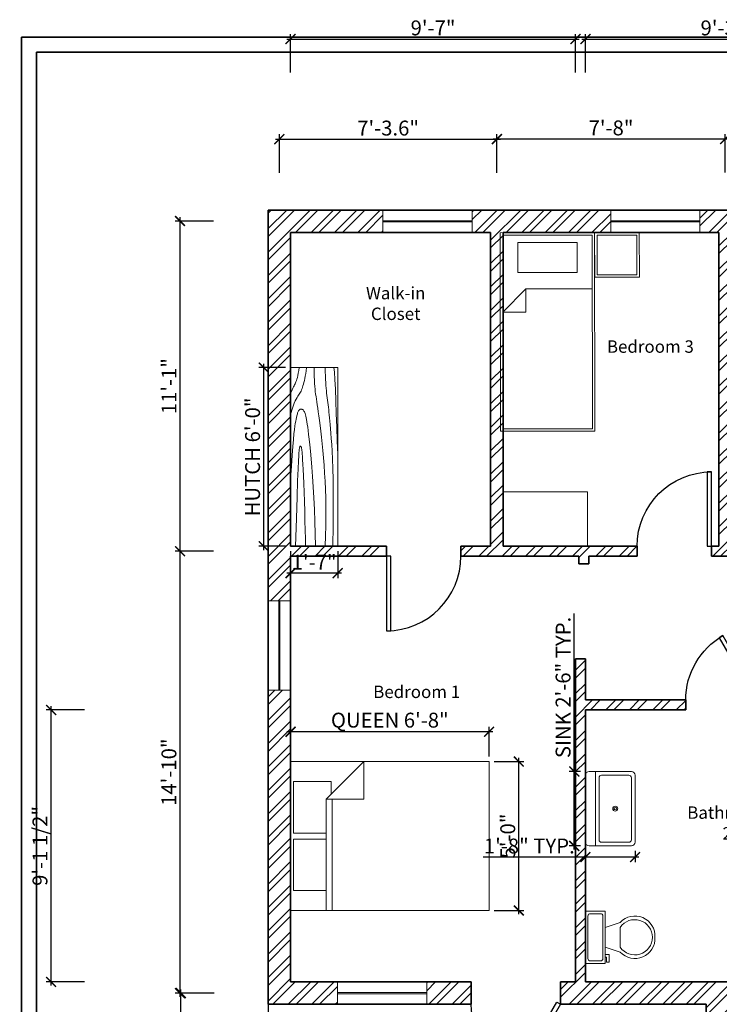
# Model space of a CAD drawing. Units: inches. Extents: x 163 to 947, y 159 to 804.
# Tile 2 of 5: x 163 to 444, y 403 to 799. Entities that reach past the tile are written whole.
import ezdxf

# ---------------------------------------------------------------- set-up
doc = ezdxf.new("R2010")
doc.units = ezdxf.units.IN
for name, color, linetype, lineweight in [('A-ANNO-TTLB', 7, 'Continuous', 35), ('A-AREA-IDEN', 7, 'Continuous', 18), ('A-FLOR-FIXT', 121, 'Continuous', 18), ('A-FLOR-OTLN', 7, 'Continuous', 25), ('Dimensions', 7, 'Continuous', 18), ('Doors', 160, 'Continuous', 25), ('Furniture', 40, 'Continuous', 18), ('Wall Hatch', 214, 'Continuous', 13), ('Walls', 222, 'Continuous', 35), ('Windows', 132, 'Continuous', 18)]:
    doc.layers.add(name, color=color, linetype=linetype, lineweight=lineweight)
doc.styles.get("Standard").update_dxf_attribs({"font": 'arial.ttf'})
doc.dimstyles.new('ISO-25', dxfattribs={"dimtxt": 6, "dimasz": 4, "dimexe": 2, "dimexo": 2, "dimtad": 1, "dimdec": 1, "dimlunit": 3, "dimtxsty": 'Standard', "dimblk": 'ARCHTICK', "dimcen": 0, "dimdle": 1.5, "dimadec": 0, "dimazin": 0, "dimtfac": 1, "dimtdec": 1, "dimtmove": 0, "dimatfit": 3, "dimfxl": 13.5, "dimfxlon": 1, "dimarcsym": 0})

# ---------------------------------------------------------------- blocks, each defined once
blk = doc.blocks.new('_ArchTick')
at = {"color": 0, "linetype": 'ByBlock', "const_width": 0.15}
blk.add_lwpolyline([(-0.5, -0.5), (0.5, 0.5)], dxfattribs=at)
blk = doc.blocks.new('*D6')
at = {"layer": 'Dimensions', "color": 0, "lineweight": -2, "transparency": 16777216}
for p, q in [((448.3, 751.36), (353.3, 751.36)), ((354.8, 737.86), (354.8, 753.36)), ((446.8, 737.86), (446.8, 753.36))]:
    blk.add_line(p, q, dxfattribs=at)
at = {"layer": 'Dimensions', "color": 0, "lineweight": -2, "transparency": 16777216, "xscale": 4, "yscale": 4, "zscale": 4, "rotation": 180}
blk.add_blockref('_ArchTick', (354.8, 751.36), dxfattribs=at)
at = {"layer": 'Dimensions', "color": 0, "lineweight": -2, "transparency": 16777216, "xscale": 4, "yscale": 4, "zscale": 4}
blk.add_blockref('_ArchTick', (446.8, 751.36), dxfattribs=at)
at = {"layer": 'Dimensions', "color": 0, "transparency": 16777216, "insert": (400.8, 755.05), "char_height": 6, "attachment_point": 5}
blk.add_mtext('7\'-8"', dxfattribs=at)
blk = doc.blocks.new('*D7')
at = {"layer": 'Dimensions', "color": 0, "lineweight": -2, "transparency": 16777216}
for p, q in [((265.66, 751.3), (356.3, 751.3)), ((267.16, 737.8), (267.16, 753.3)), ((354.8, 737.8), (354.8, 753.3))]:
    blk.add_line(p, q, dxfattribs=at)
at = {"layer": 'Dimensions', "color": 0, "lineweight": -2, "transparency": 16777216, "xscale": 4, "yscale": 4, "zscale": 4, "rotation": 180}
blk.add_blockref('_ArchTick', (267.16, 751.3), dxfattribs=at)
at = {"layer": 'Dimensions', "color": 0, "lineweight": -2, "transparency": 16777216, "xscale": 4, "yscale": 4, "zscale": 4}
blk.add_blockref('_ArchTick', (354.8, 751.3), dxfattribs=at)
at = {"layer": 'Dimensions', "color": 0, "transparency": 16777216, "insert": (310.98, 754.99), "char_height": 6, "attachment_point": 5}
blk.add_mtext('7\'-3.6"', dxfattribs=at)
blk = doc.blocks.new('*D15')
at = {"layer": 'Dimensions', "color": 0, "lineweight": -2, "transparency": 16777216}
for p, q in [((227.45, 288.78), (227.45, 408.78)), ((240.95, 407.28), (225.45, 407.28)), ((240.95, 290.28), (225.45, 290.28))]:
    blk.add_line(p, q, dxfattribs=at)
at = {"layer": 'Dimensions', "color": 0, "lineweight": -2, "transparency": 16777216, "xscale": 4, "yscale": 4, "zscale": 4}
for p, rotation in [((227.45, 407.28), 90), ((227.45, 290.28), 270)]:
    blk.add_blockref('_ArchTick', p, dxfattribs=dict(at, rotation=rotation))
at = {"layer": 'Dimensions', "color": 0, "transparency": 16777216, "insert": (223.76, 348.78), "char_height": 6, "attachment_point": 5, "rotation": 90}
blk.add_mtext('9\'-9"', dxfattribs=at)
blk = doc.blocks.new('*D16')
at = {"layer": 'Dimensions', "color": 0, "lineweight": -2, "transparency": 16777216}
for p, q in [((240.62, 585.28), (225.12, 585.28)), ((227.12, 405.78), (227.12, 586.78)), ((240.62, 407.28), (225.12, 407.28))]:
    blk.add_line(p, q, dxfattribs=at)
at = {"layer": 'Dimensions', "color": 0, "lineweight": -2, "transparency": 16777216, "xscale": 4, "yscale": 4, "zscale": 4}
for p, rotation in [((227.12, 585.28), 90), ((227.12, 407.28), 270)]:
    blk.add_blockref('_ArchTick', p, dxfattribs=dict(at, rotation=rotation))
at = {"layer": 'Dimensions', "color": 0, "transparency": 16777216, "insert": (223.43, 496.28), "char_height": 6, "attachment_point": 5, "rotation": 90}
blk.add_mtext('14\'-10"', dxfattribs=at)
blk = doc.blocks.new('*D17')
at = {"layer": 'Dimensions', "color": 0, "lineweight": -2, "transparency": 16777216}
for p, q in [((240.62, 718.32), (225.12, 718.32)), ((227.12, 583.78), (227.12, 719.82)), ((240.62, 585.28), (225.12, 585.28))]:
    blk.add_line(p, q, dxfattribs=at)
at = {"layer": 'Dimensions', "color": 0, "lineweight": -2, "transparency": 16777216, "xscale": 4, "yscale": 4, "zscale": 4}
for p, rotation in [((227.12, 718.32), 90), ((227.12, 585.28), 270)]:
    blk.add_blockref('_ArchTick', p, dxfattribs=dict(at, rotation=rotation))
at = {"layer": 'Dimensions', "color": 0, "transparency": 16777216, "insert": (223.48, 651.8), "char_height": 6, "attachment_point": 5, "rotation": 90}
blk.add_mtext('11\'-1"', dxfattribs=at)
blk = doc.blocks.new('*U19')
for p, q in [((0, 0), (0, 4)), ((30, 0), (30, 4))]:
    blk.add_line(p, q)
blk.add_lwpolyline([(0, 0), (0, -30), (1.75, -30), (1.75, 0)], close=True)
blk.add_arc((0, 0), 30, 270, 0)
blk = doc.blocks.new('*U20')
for p, q in [((0, 0), (0, -4)), ((30, 0), (30, -4))]:
    blk.add_line(p, q)
blk.add_lwpolyline([(0, 0), (0, 30), (1.75, 30), (1.75, 0)], close=True)
blk.add_arc((0, 0), 30, 0, 90)
blk = doc.blocks.new('*U21')
for p, q in [((0, 0), (0, -4)), ((30, 0), (30, -4))]:
    blk.add_line(p, q)
blk.add_lwpolyline([(0, 0), (15, 25.98), (16.52, 25.11), (1.52, -0.87)], close=True)
blk.add_arc((0, 0), 30, 0, 60)
blk = doc.blocks.new('*U22')
for p, q in [((0, 0), (0, 6)), ((36, 0), (36, 6))]:
    blk.add_line(p, q)
blk.add_lwpolyline([(0, 0), (18, -31.18), (19.52, -30.3), (1.52, 0.88)], close=True)
blk.add_arc((0, 0), 36, 300, 0)
blk = doc.blocks.new('Bed - Queen')
for p, q in [((0, -80.00003), (0, 0)), ((0, 0), (59.99999, 0)), ((59.99999, 0), (59.99999, -80.00003)), ((7.99999, -1.2), (28.79998, -1.2)), ((7.99999, -14.4), (7.99999, -1.2)), ((28.79998, -1.2), (28.79998, -14.4)), ((31.19999, -1.2), (51.99999, -1.2)), ((31.19999, -14.4), (31.19999, -1.2)), ((51.99999, -1.2), (51.99999, -16.4)), ((0, -14.4), (44.8, -14.4)), ((59.99999, -29.6), (44.8, -14.4)), ((44.8, -14.4), (44.8, -29.6)), ((44.8, -16.8), (0, -16.8)), ((51.99999, -16.4), (46.79936, -16.4)), ((44.8, -29.6), (59.99999, -29.6)), ((59.99999, -80.00003), (0, -80.00003))]:
    blk.add_line(p, q)
blk = doc.blocks.new('Hutch - 19 x 72 in.')
for p, q in [((0, -19), (0, 0)), ((0, 0), (71.999994, 0)), ((71.999994, 0), (71.999994, -19)), ((71.999994, -19), (0, -19))]:
    blk.add_line(p, q)
for points in [[(26.99999, 0), (32.30411, -0.35238), (36.66731, -0.66276), (40.20336, -0.93603), (43.02603, -1.17708), (45.2491, -1.39079), (46.98632, -1.58203), (48.35147, -1.7557), (49.45833, -1.91667), (50.40388, -2.06917), (51.21809, -2.21484), (51.91414, -2.35465), (52.5052, -2.48958), (53.00447, -2.6206), (53.42512, -2.7487), (53.78035, -2.87484), (54.08333, -3), (54.34537, -3.12516), (54.57031, -3.2513), (54.76008, -3.37939), (54.91666, -3.51042), (55.04198, -3.64534), (55.13801, -3.78516), (55.2067, -3.93083), (55.24999, -4.08333), (55.26904, -4.24316), (55.26171, -4.40885), (55.22509, -4.57845), (55.15624, -4.75), (55.05224, -4.92155), (54.91015, -5.09115), (54.72704, -5.25684), (54.49999, -5.41667), (54.22493, -5.56934), (53.89322, -5.71615), (53.49511, -5.85905), (53.02083, -6), (52.4606, -6.14095), (51.80468, -6.28385), (51.04329, -6.43066), (50.16666, -6.58333), (49.16007, -6.74381), (47.98892, -6.91406), (46.61368, -7.09603), (44.99478, -7.29167), (43.09268, -7.50293), (40.86783, -7.73177), (38.28067, -7.98014), (35.29166, -8.25), (31.87654, -8.54053), (28.07226, -8.83984), (23.93107, -9.1333), (19.5052, -9.40625), (14.84692, -9.64404), (10.00846, -9.83203), (5.04207, -9.95557), (0, -10)], [(52.99999, 0), (54.87133, -0.53955), (56.39257, -1.03516), (57.61205, -1.48975), (58.57812, -1.90625), (59.3391, -2.2876), (59.94335, -2.63672), (60.4392, -2.95654), (60.87499, -3.25), (61.29247, -3.52002), (61.70702, -3.76953), (62.12743, -4.00146), (62.56249, -4.21875), (63.02099, -4.42432), (63.51171, -4.62109), (64.04345, -4.81201), (64.62499, -5), (65.26489, -5.1875), (65.9707, -5.375), (66.74975, -5.5625), (67.60937, -5.75), (68.55688, -5.9375), (69.5996, -6.125), (70.744867, -6.3125), (71.999994, -6.5)], [(61.49999, 0), (62.35961, -0.35254), (63.08007, -0.66406), (63.68627, -0.94043), (64.20312, -1.1875), (64.65551, -1.41113), (65.06835, -1.61719), (65.46655, -1.81152), (65.87499, -2), (66.31762, -2.1875), (66.81445, -2.375), (67.38452, -2.5625), (68.04687, -2.75), (68.82055, -2.9375), (69.7246, -3.125), (70.77807, -3.3125), (71.999994, -3.5)], [(0, -2), (11.2006, -2.34123), (19.90169, -2.62044), (26.43969, -2.84595), (31.15103, -3.02604), (34.37214, -3.16903), (36.43945, -3.2832), (37.68936, -3.37687), (38.45833, -3.45833), (39.02937, -3.53459), (39.472, -3.60742), (39.80232, -3.67733), (40.03645, -3.74479), (40.1905, -3.8103), (40.28059, -3.87435), (40.32283, -3.93742), (40.33333, -4), (40.32405, -4.0625), (40.29036, -4.125), (40.22346, -4.1875), (40.11458, -4.25), (39.95491, -4.3125), (39.73567, -4.375), (39.44807, -4.4375), (39.08333, -4.5), (38.62491, -4.56282), (38.02538, -4.6276), (37.22957, -4.69629), (36.18228, -4.77083), (34.82836, -4.85319), (33.11262, -4.94531), (30.97989, -5.04915), (28.37499, -5.16667), (25.27416, -5.29818), (21.77929, -5.4375), (18.02368, -5.57682), (14.14062, -5.70833), (10.26342, -5.82422), (6.52539, -5.91667), (3.05981, -5.97786), (0, -6)], [(71.999994, -9.5), (70.071934, -9.51147), (68.38801, -9.54492), (66.91113, -9.59888), (65.60416, -9.67187), (64.43001, -9.76245), (63.35156, -9.86914), (62.3317, -9.99048), (61.33333, -10.125), (60.32128, -10.27157), (59.26822, -10.43034), (58.14876, -10.60181), (56.93749, -10.78646), (55.60904, -10.98478), (54.13801, -11.19726), (52.49902, -11.4244), (50.66666, -11.66667), (48.62239, -11.92358), (46.37499, -12.19075), (43.9401, -12.46281), (41.33333, -12.73437), (38.57031, -13.00008), (35.66666, -13.25456), (32.63801, -13.49243), (29.49999, -13.70833), (26.26367, -13.89689), (22.92187, -14.05273), (19.46289, -14.17049), (15.875, -14.24479), (12.14648, -14.27026), (8.26562, -14.24154), (4.2207, -14.15324), (0, -14)], [(0, -17), (8.37556, -17.14274), (15.58268, -17.20443), (21.74194, -17.19775), (26.97395, -17.13542), (31.39933, -17.03011), (35.13866, -16.89453), (38.31257, -16.74137), (41.04166, -16.58333), (43.4322, -16.43083), (45.5332, -16.28516), (47.37931, -16.14534), (49.0052, -16.01042), (50.44555, -15.87939), (51.73502, -15.7513), (52.90828, -15.62516), (53.99999, -15.5), (55.04044, -15.37508), (56.04231, -15.25065), (57.01391, -15.1272), (57.96353, -15.00521), (58.89949, -14.88517), (59.83007, -14.76758), (60.76358, -14.65291), (61.70833, -14.54167), (62.6752, -14.43465), (63.68554, -14.33398), (64.76326, -14.24211), (65.93229, -14.16146), (67.21655, -14.09448), (68.63997, -14.04362), (70.226475, -14.01131), (71.999994, -14)], [(36.99999, -19), (42.40038, -18.8125), (47.95312, -18.625), (53.43554, -18.4375), (58.62499, -18.25), (63.29882, -18.0625), (67.23437, -17.875), (70.208978, -17.6875), (71.999994, -17.5)]]:
    blk.add_lwpolyline(points)
blk = doc.blocks.new('*U50')
for p, q in [((9.5, -6), (9.5, -2)), ((-10, -8.5), (-8, -8.5)), ((-10, -9.5), (-10, -8.5)), ((-7, -9.5), (-10, -9.5)), ((-8, -8.5), (-8, -8)), ((-7, -8), (-7, -9.5)), ((-4, -8), (-6, -14)), ((4, -8), (6, -14)), ((4, -14), (-4, -14))]:
    blk.add_line(p, q)
blk.add_lwpolyline([(10.5, -8), (10.5, 0), (-10.5, 0), (-10.5, -8)], close=True)
for points in [[(-9.5, -2), (-9.5, -6)], [(8.5, -1), (-8.5, -1)], [(-8.5, -7), (8.5, -7)]]:
    blk.add_lwpolyline(points)
for centre, radius, start, end in [((-8.625, -1.875), 0.8839, 81.8699, 188.1301), ((8.625, -1.875), 0.8839, 351.8699, 98.1301), ((-8.625, -6.125), 0.8839, 171.869898, 278.1301), ((8.625, -6.125), 0.8839, 261.8699, 8.1301), ((-0.4772, -19.9188), 8.0953, 133.01722, 273.38), ((0.0374, -19.8731), 7.127, 124.50543, 269.7), ((-0.0373, -19.8731), 7.127, 270.3, 55.4946), ((0.4773, -19.9188), 8.0953, 266.62, 46.9828)]:
    blk.add_arc(centre, radius, start, end)
blk = doc.blocks.new('Sink-single - 30 in top')
blk.add_line((-15, -3.999996), (15, -3.999996))
for points in [[(-13.5, 0), (13.5, 0)], [(-15, -18.499996), (-15, -1.5)], [(15, -1.5), (15, -18.499996)], [(-13.5, -17.499996), (-13.5, -6.499996)], [(-12.5, -5.499996), (12.5, -5.499996)], [(13.5, -6.499996), (13.5, -17.499996)], [(12.5, -18.499996), (-12.5, -18.499996)], [(13.5, -19.999996), (-13.5, -19.999996)]]:
    blk.add_lwpolyline(points)
for radius in [1, 0.5]:
    blk.add_circle((0, -11.999996), radius)
for centre, radius, start, end in [((-13.5, -1.5), 1.5, 90, 180), ((13.5, -1.5), 1.5, 0, 90), ((-12.5, -6.499996), 1, 90, 180), ((12.5, -6.499996), 1, 0, 90), ((-13.5, -18.499996), 1.5, 180, 270), ((-12.5, -17.499996), 1, 180, 270), ((12.5, -17.499996), 1, 270, 0), ((13.5, -18.499996), 1.5, 270, 0)]:
    blk.add_arc(centre, radius, start, end)
blk = doc.blocks.new('WIN-36IN')
for p, q in [((0, 9.03), (0, 0)), ((35.98, 9.03), (35.98, 0)), ((0, 4.76), (35.98, 4.76)), ((0, 4.26), (35.98, 4.26))]:
    blk.add_line(p, q)
blk = doc.blocks.new('BED-TWIN')
for p, q in [((1, 57.33), (27.7, 57.33)), ((27.7, 57.33), (37, 48.04)), ((27.7, 48.04), (27.7, 57.33)), ((37, 48.04), (27.7, 48.04))]:
    blk.add_line(p, q)
for points in [[(0, 0), (38, 0), (38, 80), (0, 80)], [(1, 1), (37, 1), (37, 79), (1, 79)], [(7, 64), (31, 64), (31, 76), (7, 76)]]:
    blk.add_lwpolyline(points, close=True)
blk = doc.blocks.new('NIGHTSTAND-18IN')
for points in [[(0, 0), (18, 0), (18, 18), (0, 18)], [(1, 1), (17, 1), (17, 17), (1, 17)]]:
    blk.add_lwpolyline(points, close=True)
blk = doc.blocks.new('BEDROOM-CABINET-34X22')
blk.add_lwpolyline([(0, 0), (34, 0), (34, 22), (0, 22)], close=True)
blk = doc.blocks.new('*D66')
at = {"layer": 'Dimensions', "color": 0, "lineweight": -2, "transparency": 16777216}
for p, q in [((386, 496.57), (386, 560.26)), ((388.5, 496.57), (384, 496.57)), ((386, 465.07), (386, 496.57)), ((388.5, 466.57), (384, 466.57))]:
    blk.add_line(p, q, dxfattribs=at)
at = {"layer": 'Dimensions', "color": 0, "lineweight": -2, "transparency": 16777216, "xscale": 4, "yscale": 4, "zscale": 4}
for p, rotation in [((386, 496.57), 90), ((386, 466.57), 270)]:
    blk.add_blockref('_ArchTick', p, dxfattribs=dict(at, rotation=rotation))
at = {"layer": 'Dimensions', "color": 0, "transparency": 16777216, "insert": (382.27, 530.42), "char_height": 6, "attachment_point": 5, "rotation": 90}
blk.add_mtext('SINK 2\'-6" TYP.', dxfattribs=at)
blk = doc.blocks.new('*D67')
at = {"layer": 'Dimensions', "color": 0, "lineweight": -2, "transparency": 16777216}
for p, q in [((390.5, 464.57), (390.5, 460.07)), ((410.5, 464.57), (410.5, 460.07)), ((390.5, 462.07), (349.24, 462.07)), ((412, 462.07), (390.5, 462.07))]:
    blk.add_line(p, q, dxfattribs=at)
at = {"layer": 'Dimensions', "color": 0, "lineweight": -2, "transparency": 16777216, "xscale": 4, "yscale": 4, "zscale": 4, "rotation": 180}
blk.add_blockref('_ArchTick', (390.5, 462.07), dxfattribs=at)
at = {"layer": 'Dimensions', "color": 0, "lineweight": -2, "transparency": 16777216, "xscale": 4, "yscale": 4, "zscale": 4}
blk.add_blockref('_ArchTick', (410.5, 462.07), dxfattribs=at)
at = {"layer": 'Dimensions', "color": 0, "transparency": 16777216, "insert": (367.87, 465.76), "char_height": 6, "attachment_point": 5}
blk.add_mtext('1\'-8" TYP.', dxfattribs=at)
blk = doc.blocks.new('*D82')
at = {"layer": 'Dimensions', "color": 0, "lineweight": -2, "transparency": 16777216}
for p, q in [((353.16, 512.56), (270.16, 512.56)), ((271.66, 502.56), (271.66, 514.56)), ((351.66, 502.56), (351.66, 514.56))]:
    blk.add_line(p, q, dxfattribs=at)
at = {"layer": 'Dimensions', "color": 0, "lineweight": -2, "transparency": 16777216, "xscale": 4, "yscale": 4, "zscale": 4, "rotation": 180}
blk.add_blockref('_ArchTick', (271.66, 512.56), dxfattribs=at)
at = {"layer": 'Dimensions', "color": 0, "lineweight": -2, "transparency": 16777216, "xscale": 4, "yscale": 4, "zscale": 4}
blk.add_blockref('_ArchTick', (351.66, 512.56), dxfattribs=at)
at = {"layer": 'Dimensions', "color": 0, "transparency": 16777216, "insert": (311.66, 516.47), "char_height": 6, "attachment_point": 5}
blk.add_mtext('QUEEN 6\'-8"', dxfattribs=at)
blk = doc.blocks.new('*D83')
at = {"layer": 'Dimensions', "color": 0, "lineweight": -2, "transparency": 16777216}
for p, q in [((353.66, 500.56), (365.66, 500.56)), ((363.66, 439.06), (363.66, 502.06)), ((353.66, 440.56), (365.66, 440.56))]:
    blk.add_line(p, q, dxfattribs=at)
at = {"layer": 'Dimensions', "color": 0, "lineweight": -2, "transparency": 16777216, "xscale": 4, "yscale": 4, "zscale": 4}
for p, rotation in [((363.66, 500.56), 90), ((363.66, 440.56), 270)]:
    blk.add_blockref('_ArchTick', p, dxfattribs=dict(at, rotation=rotation))
at = {"layer": 'Dimensions', "color": 0, "transparency": 16777216, "insert": (359.97, 470.56), "char_height": 6, "attachment_point": 5, "rotation": 90}
blk.add_mtext('5\'-0"', dxfattribs=at)
blk = doc.blocks.new('*D86')
at = {"layer": 'Dimensions', "color": 0, "lineweight": -2, "transparency": 16777216}
for p, q in [((269.66, 659.28), (258.86, 659.28)), ((260.86, 585.78), (260.86, 660.78)), ((269.66, 587.28), (258.86, 587.28))]:
    blk.add_line(p, q, dxfattribs=at)
at = {"layer": 'Dimensions', "color": 0, "lineweight": -2, "transparency": 16777216, "xscale": 4, "yscale": 4, "zscale": 4}
for p, rotation in [((260.86, 659.28), 90), ((260.86, 587.28), 270)]:
    blk.add_blockref('_ArchTick', p, dxfattribs=dict(at, rotation=rotation))
at = {"layer": 'Dimensions', "color": 0, "transparency": 16777216, "insert": (257.14, 623.28), "char_height": 6, "attachment_point": 5, "rotation": 90}
blk.add_mtext('HUTCH 6\'-0"', dxfattribs=at)
blk = doc.blocks.new('*D87')
at = {"layer": 'Dimensions', "color": 0, "lineweight": -2, "transparency": 16777216}
for p, q in [((271.66, 585.28), (271.66, 574.48)), ((290.66, 585.28), (290.66, 574.48)), ((292.16, 576.48), (270.16, 576.48))]:
    blk.add_line(p, q, dxfattribs=at)
at = {"layer": 'Dimensions', "color": 0, "lineweight": -2, "transparency": 16777216, "xscale": 4, "yscale": 4, "zscale": 4, "rotation": 180}
blk.add_blockref('_ArchTick', (271.66, 576.48), dxfattribs=at)
at = {"layer": 'Dimensions', "color": 0, "lineweight": -2, "transparency": 16777216, "xscale": 4, "yscale": 4, "zscale": 4}
blk.add_blockref('_ArchTick', (290.66, 576.48), dxfattribs=at)
at = {"layer": 'Dimensions', "color": 0, "transparency": 16777216, "insert": (281.16, 580.12), "char_height": 6, "attachment_point": 5}
blk.add_mtext('1\'-7"', dxfattribs=at)
blk = doc.blocks.new('*D90')
at = {"layer": 'Dimensions', "color": 0, "lineweight": -2, "transparency": 16777216}
for p, q in [((271.66, 778.15), (271.66, 793.65)), ((386.49, 778.15), (386.49, 793.65)), ((270.16, 791.65), (387.99, 791.65))]:
    blk.add_line(p, q, dxfattribs=at)
at = {"layer": 'Dimensions', "color": 0, "lineweight": -2, "transparency": 16777216, "xscale": 4, "yscale": 4, "zscale": 4, "rotation": 180}
blk.add_blockref('_ArchTick', (271.66, 791.65), dxfattribs=at)
at = {"layer": 'Dimensions', "color": 0, "lineweight": -2, "transparency": 16777216, "xscale": 4, "yscale": 4, "zscale": 4}
blk.add_blockref('_ArchTick', (386.49, 791.65), dxfattribs=at)
at = {"layer": 'Dimensions', "color": 0, "transparency": 16777216, "insert": (329.08, 795.34), "char_height": 6, "attachment_point": 5}
blk.add_mtext('9\'-7"', dxfattribs=at)
blk = doc.blocks.new('*D91')
at = {"layer": 'Dimensions', "color": 0, "lineweight": -2, "transparency": 16777216}
for p, q in [((390.5, 778.15), (390.5, 793.65)), ((501.32, 778.15), (501.32, 793.65)), ((389, 791.65), (502.82, 791.65))]:
    blk.add_line(p, q, dxfattribs=at)
at = {"layer": 'Dimensions', "color": 0, "lineweight": -2, "transparency": 16777216, "xscale": 4, "yscale": 4, "zscale": 4, "rotation": 180}
blk.add_blockref('_ArchTick', (390.5, 791.65), dxfattribs=at)
at = {"layer": 'Dimensions', "color": 0, "lineweight": -2, "transparency": 16777216, "xscale": 4, "yscale": 4, "zscale": 4}
blk.add_blockref('_ArchTick', (501.32, 791.65), dxfattribs=at)
at = {"layer": 'Dimensions', "color": 0, "transparency": 16777216, "insert": (445.91, 795.34), "char_height": 6, "attachment_point": 5}
blk.add_mtext('9\'-3"', dxfattribs=at)
blk = doc.blocks.new('*D92')
at = {"layer": 'Dimensions', "color": 0, "lineweight": -2, "transparency": 16777216}
for p, q in [((188.69, 521.35), (173.19, 521.35)), ((175.19, 410.29), (175.19, 522.85)), ((188.69, 411.79), (173.19, 411.79))]:
    blk.add_line(p, q, dxfattribs=at)
at = {"layer": 'Dimensions', "color": 0, "lineweight": -2, "transparency": 16777216, "xscale": 4, "yscale": 4, "zscale": 4}
for p, rotation in [((175.19, 521.35), 90), ((175.19, 411.79), 270)]:
    blk.add_blockref('_ArchTick', p, dxfattribs=dict(at, rotation=rotation))
at = {"layer": 'Dimensions', "color": 0, "transparency": 16777216, "insert": (171.47, 466.57), "char_height": 6, "attachment_point": 5, "rotation": 90}
blk.add_mtext('9\'-1 1/2"', dxfattribs=at)

msp = doc.modelspace()

# ---------------------------------------------------------------- hatches: boundary and pattern name
at = {"layer": 'Wall Hatch'}
h = msp.add_hatch(dxfattribs=at)
h.set_pattern_fill('ANSI32', color=256, scale=0.7)
h.paths.add_polyline_path([(271.66, 713.71), (308.91, 713.71), (308.91, 722.73), (262.64, 722.73), (262.64, 565.31), (271.66, 565.31), (271.66, 583.27), (310.31, 583.27), (310.31, 587.28), (271.66, 587.28)])
h.paths.add_polyline_path([(357.32, 713.71), (400.68, 713.71), (400.68, 722.73), (344.89, 722.73), (344.89, 713.71), (352.3, 713.71), (352.3, 587.28), (340.31, 587.28), (340.31, 583.27), (387.9, 583.27), (387.9, 580.28), (391.92, 580.28), (391.92, 583.27), (411.3, 583.27), (411.3, 587.28), (357.32, 587.28)])
h.paths.add_polyline_path([(454.65, 722.73), (436.66, 722.73), (436.66, 713.71), (444.3, 713.71), (444.3, 587.28), (441.3, 587.28), (441.3, 583.27), (452.32, 583.27), (452.32, 587.28), (449.32, 587.28), (449.32, 713.71), (454.65, 713.71)])
h.paths.add_polyline_path([(546.44, 722.73), (490.63, 722.73), (490.63, 713.71), (537.42, 713.71), (537.42, 587.28), (482.32, 587.28), (482.32, 583.27), (546.44, 583.27), (546.44, 630.27), (552.44, 630.27), (552.44, 639.3), (546.44, 639.3)])
h.paths.add_polyline_path([(271.66, 529.33), (262.64, 529.33), (262.64, 402.77), (290.54, 402.77), (290.54, 411.79), (271.66, 411.79)])
h.paths.add_polyline_path([(344.49, 408.77), (344.51, 411.79), (326.52, 411.79), (326.52, 402.77), (344.49, 402.77)])
h.paths.add_polyline_path([(528.33, 411.79), (510.34, 411.79), (510.34, 521.35), (546.44, 521.35), (546.44, 525.36), (460.92, 525.36), (460.9, 525.35), (460.9, 521.35), (501.32, 521.35), (501.32, 411.79), (390.5, 411.79), (390.5, 521.35), (430.9, 521.35), (430.9, 525.36), (390.5, 525.36), (390.5, 541.96), (386.49, 541.96), (386.49, 411.79), (380.49, 411.79), (380.49, 402.77), (439.11, 402.77), (439.11, 392.26), (448.14, 392.26), (448.14, 402.77), (528.33, 402.77)])
h.paths.add_polyline_path([(448.14, 356.28), (439.11, 356.28), (439.11, 338.29), (448.14, 338.29)])
h.paths.add_polyline_path([(542.45, 294.79), (448.14, 294.79), (448.14, 302.31), (439.11, 302.31), (439.11, 285.77), (542.45, 285.77)])
h.paths.add_polyline_path([(596.42, 294.79), (578.43, 294.79), (578.43, 285.77), (596.42, 285.77)])
h.paths.add_polyline_path([(653.12, 402.77), (659.11, 402.77), (659.11, 408.77), (659.11, 411.79), (626.1, 411.79), (626.1, 402.77), (644.09, 402.77), (644.09, 294.79), (632.4, 294.79), (632.4, 285.77), (653.12, 285.77)])
h.paths.add_polyline_path([(738.49, 630.27), (844.6, 630.27), (844.6, 603.27), (853.62, 603.27), (853.62, 722.73), (663.29, 722.73), (663.29, 677.29), (672.32, 677.29), (672.32, 713.71), (777.6, 713.71), (777.6, 669.29), (783.62, 669.29), (783.62, 713.71), (844.6, 713.71), (844.6, 636.29), (783.62, 636.29), (783.62, 639.29), (777.6, 639.29), (777.6, 636.29), (672.32, 636.29), (672.32, 645.29), (663.29, 645.29), (663.29, 639.3), (582.43, 639.3), (582.43, 630.27), (643.22, 630.27), (643.22, 624.27), (648.23, 624.27), (648.23, 630.27), (732.47, 630.27), (732.47, 547.43), (648.23, 547.43), (648.23, 594.27), (643.22, 594.27), (643.22, 525.36), (625.17, 525.36), (625.17, 517.34), (648.23, 517.34), (648.23, 541.41), (729.47, 541.41), (729.47, 517.34), (738.49, 517.34)])
h.paths.add_polyline_path([(853.62, 567.29), (844.6, 567.29), (844.6, 489.33), (853.62, 489.33)])
h.paths.add_polyline_path([(853.62, 453.35), (844.6, 453.35), (844.6, 411.79), (826.3, 411.79), (826.3, 402.77), (853.62, 402.77)])
h.paths.add_polyline_path([(790.32, 411.79), (772.33, 411.79), (772.33, 402.77), (790.32, 402.77)])
h.paths.add_polyline_path([(736.35, 411.79), (695.11, 411.79), (695.11, 402.77), (736.35, 402.77)])

# ---------------------------------------------------------------- linework, layer by layer
at = {"layer": 'A-ANNO-TTLB'}
for points in [[(163.29, 792.35), (947.45, 792.35), (947.45, 158.54), (163.29, 158.54)], [(169.29, 786.35), (941.45, 786.35), (941.45, 164.54), (169.29, 164.54)]]:
    msp.add_lwpolyline(points, close=True, dxfattribs=at)
at = {"layer": 'A-FLOR-OTLN'}
msp.add_line((262.64, 402.77), (262.64, 285.77), dxfattribs=at)
at = {"layer": 'Walls'}
for p, q in [((262.64, 722.73), (262.64, 402.77)), ((546.44, 722.73), (262.64, 722.73)), ((352.3, 713.71), (271.66, 713.71)), ((271.66, 713.71), (271.66, 587.28)), ((352.3, 713.71), (352.3, 587.28)), ((357.32, 713.71), (357.32, 587.28)), ((444.3, 713.71), (357.32, 713.71)), ((444.3, 713.71), (444.3, 587.28)), ((310.31, 587.28), (271.66, 587.28)), ((310.31, 587.28), (310.31, 583.27)), ((352.3, 587.28), (340.31, 587.28)), ((340.31, 587.28), (340.31, 583.27)), ((411.3, 587.28), (357.32, 587.28)), ((411.3, 587.28), (411.3, 583.27)), ((444.3, 587.28), (441.3, 587.28)), ((441.3, 587.28), (441.3, 583.27)), ((310.31, 583.27), (271.66, 583.27)), ((271.66, 583.27), (271.66, 411.79)), ((387.9, 583.27), (340.31, 583.27)), ((387.9, 583.27), (387.9, 580.28)), ((391.92, 583.27), (391.92, 580.28)), ((411.3, 583.27), (391.92, 583.27)), ((452.32, 583.27), (441.3, 583.27)), ((387.9, 580.28), (391.92, 580.28)), ((386.49, 541.96), (390.5, 541.96)), ((386.49, 541.96), (386.49, 411.79)), ((390.5, 541.96), (390.5, 525.36)), ((430.92, 525.36), (390.5, 525.36)), ((430.92, 525.36), (430.92, 521.35)), ((430.92, 521.35), (390.5, 521.35)), ((390.5, 521.35), (390.5, 411.79)), ((344.51, 411.79), (271.66, 411.79)), ((344.51, 411.79), (344.51, 402.77)), ((386.49, 411.79), (380.49, 411.79)), ((380.49, 411.79), (380.49, 402.77)), ((501.32, 411.79), (390.5, 411.79)), ((344.51, 402.77), (262.64, 402.77)), ((439.11, 402.77), (380.49, 402.77)), ((439.11, 402.77), (439.11, 285.77))]:
    msp.add_line(p, q, dxfattribs=at)

# ---------------------------------------------------------------- block references
at = {"layer": 'A-FLOR-FIXT'}
for name, p, rotation in [('Sink-single - 30 in top', (390.5, 481.57), 90), ('*U50', (390.5, 429.77), 90.00000000000003)]:
    msp.add_blockref(name, p, dxfattribs=dict(at, rotation=rotation))
at = {"layer": 'Doors', "xscale": -1}
for name, p in [('*U20', (441.3, 587.27)), ('*U21', (460.9, 525.35)), ('*U22', (380.49, 402.77))]:
    msp.add_blockref(name, p, dxfattribs=at)
at = {"layer": 'Doors'}
msp.add_blockref('*U19', (310.31, 583.27), dxfattribs=at)
at = {"layer": 'Furniture', "extrusion": (0, 0, -1), "zscale": -1, "rotation": 359.9423208395009}
msp.add_blockref('BED-TWIN', (-394.28, 633.65), dxfattribs=at)
at = {"layer": 'Furniture'}
for name, p, rotation in [('NIGHTSTAND-18IN', (412.22, 695.67), 90.05767916049643), ('Hutch - 19 x 72 in.', (271.66, 587.28), 90), ('Bed - Queen', (271.66, 440.56), 90)]:
    msp.add_blockref(name, p, dxfattribs=dict(at, rotation=rotation))
msp.add_blockref('BEDROOM-CABINET-34X22', (357.32, 587.28), dxfattribs=at)
at = {"layer": 'Windows'}
for p in [(308.91, 713.7), (400.68, 713.7), (290.54, 402.77)]:
    msp.add_blockref('WIN-36IN', p, dxfattribs=at)
at = {"layer": 'Windows', "rotation": 90.00000000000026}
msp.add_blockref('WIN-36IN', (271.66, 529.33), dxfattribs=at)

# ---------------------------------------------------------------- texts
at = {"layer": 'A-AREA-IDEN', "char_height": 5, "attachment_point": 1}
for s, insert in [('\\pxqc;{\\fTimes New Roman|b0|i0|c0|p18;Walk-in Closet}', (295.99, 691.78)), ('\\pxqc;{\\fTimes New Roman|b0|i0|c0|p18;Bedroom 3}', (398.62, 670.24)), ('\\pxqc;{\\fTimes New Roman|b0|i0|c0|p18;Bedroom 1}', (304.45, 531.15)), ('\\pxqc;{\\fTimes New Roman|b0|i0|c0|p18;Bathroom 2}', (429.6, 482.49))]:
    msp.add_mtext_dynamic_manual_height_columns(s, width=36.0874, gutter_width=12.5, heights=[0], dxfattribs=dict(at, insert=insert))

# ---------------------------------------------------------------- dimensions: what is measured, and where the dimension line sits
at = {"layer": 'Dimensions'}
for base, p1, p2, override, picture, middle in [((386.49, 791.65), (271.66, 529.33), (386.49, 541.96), {"dimdec": 1, "dimlfac": 1, "dimrnd": 0, "dimzin": 1, "dimdsep": 46, "dimlunit": 4, "dimfrac": 2}, '*D90', (329.08, 795.34)), ((501.32, 791.65), (390.5, 521.35), (501.32, 521.35), {"dimdec": 1, "dimlfac": 1, "dimrnd": 0, "dimzin": 1, "dimdsep": 46, "dimlunit": 4, "dimfrac": 2}, '*D91', (445.91, 795.34)), ((354.8, 751.3), (267.16, 724.34), (354.8, 724.34), {"dimclrd": 0, "dimclre": 0, "dimclrt": 0}, '*D7', (310.98, 754.99)), ((354.8, 751.36), (446.8, 724.34), (354.8, 724.34), {"dimclrd": 0, "dimclre": 0, "dimclrt": 0}, '*D6', (400.8, 755.05))]:
    dim = msp.add_linear_dim(base=base, p1=p1, p2=p2, dimstyle='ISO-25', override=override, dxfattribs=at)
    dim.commit()
    dim.dimension.update_dxf_attribs({"geometry": picture, "text_midpoint": middle})
for base, p1, p2, angle, override, picture, middle in [((227.12, 718.32), (256.15, 585.28), (256.15, 718.32), 90, {"dimclrd": 0, "dimclre": 0, "dimclrt": 0}, '*D17', (223.48, 651.8)), ((227.12, 585.28), (256.15, 407.28), (256.15, 585.28), 90, {"dimclrd": 0, "dimclre": 0, "dimclrt": 0}, '*D16', (223.43, 496.28)), ((271.66, 576.48), (290.66, 587.28), (271.66, 587.28), 180, {"dimdec": 1, "dimlfac": 1, "dimrnd": 0, "dimzin": 1, "dimdsep": 46, "dimlunit": 4, "dimfrac": 2}, '*D87', (281.16, 580.12)), ((175.19, 521.35), (501.32, 411.79), (501.32, 521.35), 90, {"dimdec": 1, "dimlfac": 1, "dimrnd": 0, "dimzin": 1, "dimdsep": 46, "dimlunit": 4, "dimfrac": 2}, '*D92', (171.47, 466.57)), ((363.66, 500.56), (351.66, 440.56), (351.66, 500.56), 90, {"dimdec": 1, "dimlfac": 1, "dimrnd": 0, "dimzin": 1, "dimdsep": 46, "dimlunit": 4, "dimfrac": 2}, '*D83', (359.97, 470.56)), ((227.45, 407.28), (256.15, 290.28), (256.15, 407.28), 90, {"dimclrd": 0, "dimclre": 0, "dimclrt": 0}, '*D15', (223.76, 348.78))]:
    dim = msp.add_linear_dim(base=base, p1=p1, p2=p2, angle=angle, dimstyle='ISO-25', override=override, dxfattribs=at)
    dim.commit()
    dim.dimension.update_dxf_attribs({"geometry": picture, "text_midpoint": middle})
for base, p1, p2, angle, text, picture, middle in [((260.86, 659.28), (271.66, 587.28), (271.66, 659.28), 90, 'HUTCH <>', '*D86', (257.14, 623.28)), ((386, 496.57), (390.5, 466.57), (390.5, 496.57), 90, 'SINK <> TYP.', '*D66', (382.27, 530.42)), ((271.66, 512.56), (351.66, 500.56), (271.66, 500.56), 180, 'QUEEN <>', '*D82', (311.66, 516.47)), ((390.5, 462.07), (410.5, 466.57), (390.5, 466.57), 180, '<> TYP.', '*D67', (367.87, 465.76))]:
    dim = msp.add_linear_dim(base=base, p1=p1, p2=p2, angle=angle, text=text, dimstyle='ISO-25', override={"dimdec": 1, "dimlfac": 1, "dimrnd": 0, "dimzin": 1, "dimdsep": 46, "dimlunit": 4, "dimfrac": 2}, dxfattribs=at)
    dim.commit()
    dim.dimension.update_dxf_attribs({"geometry": picture, "text_midpoint": middle})

doc.saveas('drawing.dxf')
